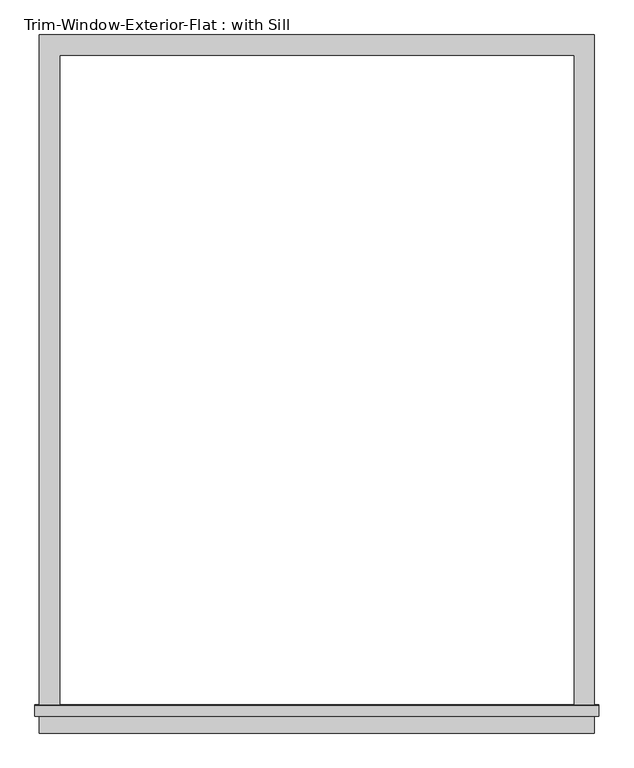
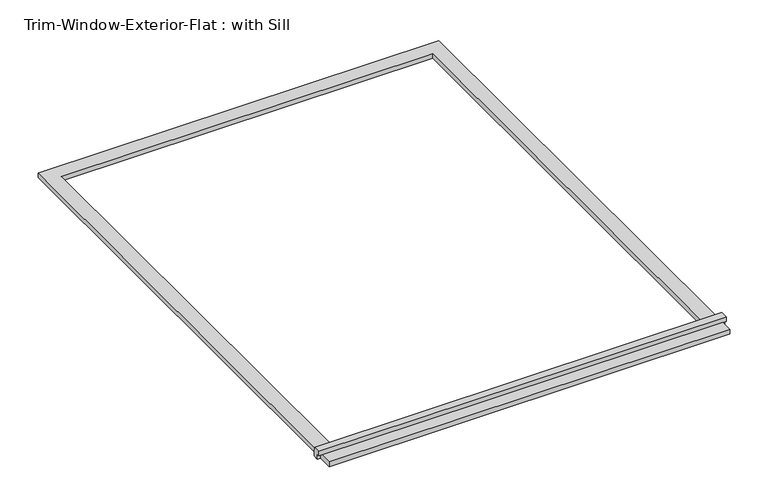
"""IFC4 building model written with IfcOpenShell, lengths in millimetres: proxy geometry, Trim-Window-Exterior-Flat : with Sill."""

from ifc_helpers import new_model, si_unit, frame, origin, origin_with_axes, place, context, project, spatial, polyline, outline, extrude, source, transform, mapped, element, save


def trim_window_exterior_flat_with_sill_e04b3088(model_context):
    return source(origin(), model_context, "Body", "SweptSolid", [
        extrude(outline(polyline([(781.05, -1850.9823709), (781.05, -1908.1323709), (-781.05, -1908.1323709), (-781.05, -1850.9823709), (781.05, -1850.9823709)])), origin_with_axes(), (0.0, 0.0, 1.0), 19.05),
        extrude(outline(polyline([(-1860.55, 38.1), (-1831.2580645, 38.1), (-1828.8, 19.05), (-1828.8, 0.0), (-1850.9823709, 0.0), (-1850.9823709, 19.05), (-1860.55, 19.05), (-1860.55, 38.1)])), frame((-793.75, 0.0, 0.0), z_axis=(1.0, 0.0, 0.0), x_axis=(0.0, 1.0, 0.0)), (0.0, 0.0, 1.0), 1587.5),
        extrude(outline(polyline([(-781.05, 57.15), (781.05, 57.15), (781.05, -1828.8), (723.9, -1828.8), (723.9, 0.0), (-723.9, 0.0), (-723.9, -1828.8), (-781.05, -1828.8), (-781.05, 57.15)])), origin_with_axes(), (0.0, 0.0, 1.0), 19.05),
    ])


if __name__ == "__main__":
    model = new_model("IFC4")
    model_context = context("Model", 3, world=origin())
    ifc_project = project(units=[si_unit("LENGTHUNIT", "METRE", prefix="MILLI")], contexts=[model_context])
    site = spatial("IfcSite", under=ifc_project)
    building = spatial("IfcBuilding", under=site)
    placement = place(None, origin())
    trim_window_exterior_flat_with_sill_shape = trim_window_exterior_flat_with_sill_e04b3088(model_context)
    element("IfcBuildingElementProxy", 1, Name="Trim-Window-Exterior-Flat : with Sill", ObjectType="Trim-Window-Exterior-Flat : with Sill", at=placement, inside=building, context=model_context, shape_type="MappedRepresentation", body=[
        mapped(trim_window_exterior_flat_with_sill_shape, transform((0.0, 0.0, 0.0), x_axis=(1.0, 0.0, 0.0), y_axis=(0.0, 1.0, 0.0), z_axis=(0.0, 0.0, 1.0))),
    ])
    save(model, "model.ifc")

# Revit data of these elements
# Type "Trim-Window-Exterior-Flat : with Sill"
#   Trim Width = 0' - 2 1/4"
#   Trim Thickness_Picture Frame = 0' - 1 1/4"
#   Trim Thickness_with Sill = 0' - 0 3/4"
#   Sill Thickness = 0' - 1 1/4"
#   Opening Width [instance default] = 2' - 0"
#   Opening Height [instance default] = 3' - 0"
#   Default Elevation = 4' - 0"
#   Sill = yes
#   Picture Frame = no
#   Trim Material [instance default] = none
# Element 1 (IfcBuildingElementProxy, "Trim-Window-Exterior-Flat : with Sill")
#   Opening Width = 4' - 9"
#   Opening Height = 6' - 0"
#   Trim Material = Clad - White
#   Materials on its faces: "Clad - White"
# Materials
#   "Clad - White": class "Wood", colour RGB 242 242 238, transparency 0, Cost = 0
